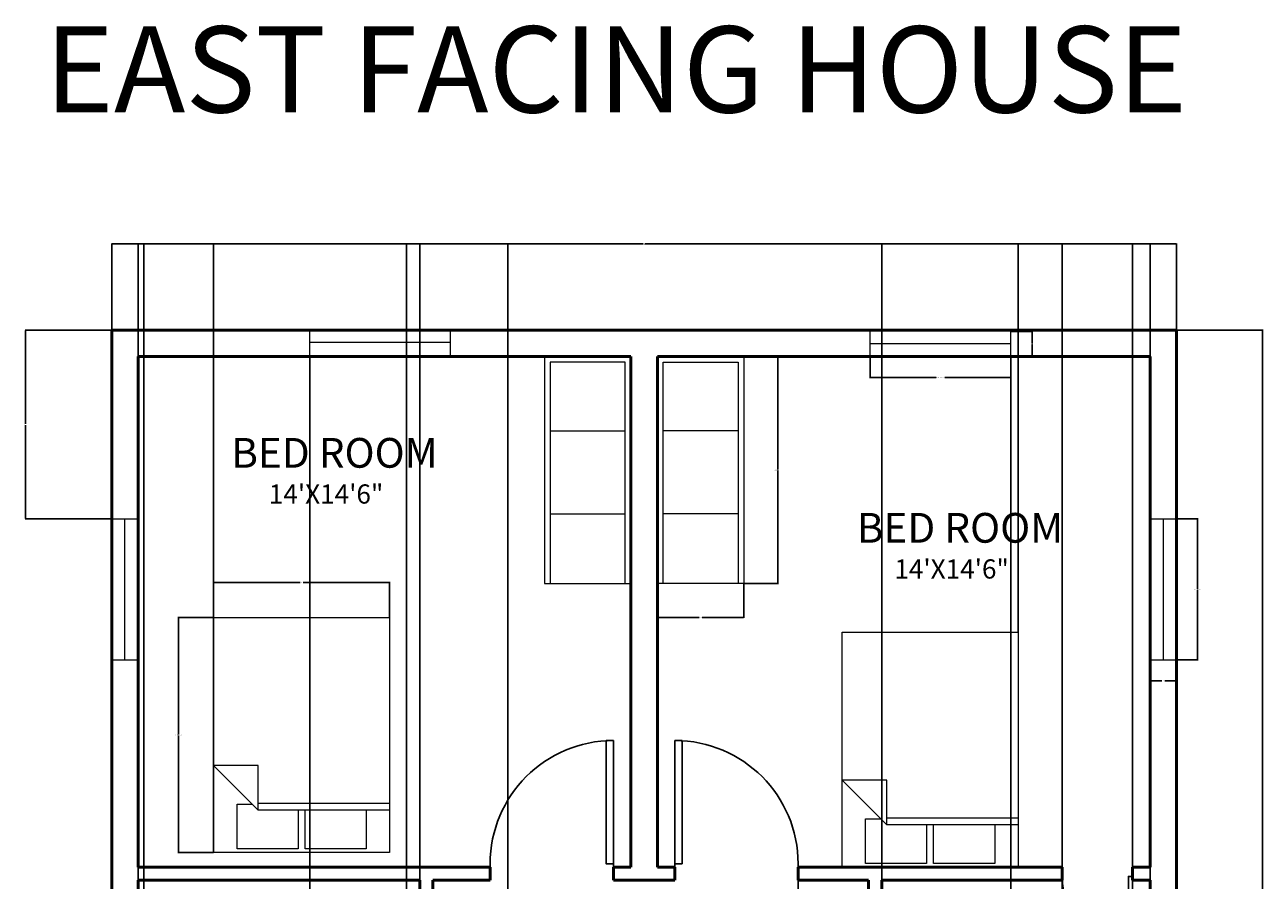
# Model space of a CAD drawing. Units: inches. Extents: x 19425 to 19848, y 45806 to 46417.
# Tile 5 of 5: x 19425 to 19847, y 46125 to 46417. Entities that reach past the tile are written whole.
import ezdxf

# ---------------------------------------------------------------- set-up
doc = ezdxf.new("R2010")
doc.units = ezdxf.units.IN
for name, color, linetype, lineweight in [('A-ANNO-DIMS', 2, 'Continuous', 18), ('A-ANNO-TITL', 7, 'Continuous', 35), ('A-AREA-IDEN', 3, 'Continuous', 25), ('A-FLOR-CASE', 2, 'Continuous', 20), ('door', 4, 'Continuous', 25), ('furniture', 2, 'Continuous', 18), ('wall', 6, 'Continuous', 50), ('window', 9, 'Continuous', 20)]:
    doc.layers.add(name, color=color, linetype=linetype, lineweight=lineweight)
doc.styles.get("Standard").update_dxf_attribs({"font": 'arial.ttf'})
doc.dimstyles.get("Standard").update_dxf_attribs({"dimtxt": 0.18, "dimasz": 0.18, "dimexe": 0.18, "dimexo": 0.0625, "dimgap": 0.09, "dimtad": 0, "dimtih": 1, "dimtoh": 1, "dimdec": 4, "dimzin": 0, "dimdsep": 46, "dimtxsty": 'Standard', "dimcen": 0.09, "dimadec": 0, "dimazin": 0, "dimtfac": 1, "dimtdec": 4, "dimtofl": 0, "dimtmove": 0, "dimatfit": 3, "dimfxl": 1, "dimtolj": 1, "dimtzin": 0, "dimarcsym": 0})

# ---------------------------------------------------------------- blocks, each defined once
blk = doc.blocks.new('*U2')
for p, q in [((0, 0), (0, -100)), ((750, 0), (750, -100))]:
    blk.add_line(p, q)
blk.add_lwpolyline([(0, 0), (0, 750), (43.75, 750), (43.75, 0)], close=True)
blk.add_arc((0, 0), 750, 0, 90)
blk = doc.blocks.new('Bed - Queen')
for p, q in [((0, -80.00003), (0, 0)), ((0, 0), (59.99999, 0)), ((59.99999, 0), (59.99999, -80.00003)), ((7.99999, -1.2), (28.79998, -1.2)), ((7.99999, -14.4), (7.99999, -1.2)), ((28.79998, -1.2), (28.79998, -14.4)), ((31.19999, -1.2), (51.99999, -1.2)), ((31.19999, -14.4), (31.19999, -1.2)), ((51.99999, -1.2), (51.99999, -16.4)), ((0, -14.4), (44.8, -14.4)), ((44.8, -16.8), (0, -16.8)), ((59.99999, -29.6), (44.8, -14.4)), ((44.8, -14.4), (44.8, -29.6)), ((51.99999, -16.4), (46.79936, -16.4)), ((44.8, -29.6), (59.99999, -29.6)), ((59.99999, -80.00003), (0, -80.00003))]:
    blk.add_line(p, q)
blk = doc.blocks.new('WIN-48-CENTER-9')
for p, q in [((0, 48), (9, 48)), ((4.5, 0), (4.5, 48)), ((0, 0), (9, 0))]:
    blk.add_line(p, q)
blk = doc.blocks.new('WIN-48-SHALLOW')
for p, q in [((0, 0), (0, 8.56)), ((48, 0), (48, 8.56)), ((48, 4.28), (0, 4.28))]:
    blk.add_line(p, q)
blk = doc.blocks.new('BEDROOM-WARDROBE')
for p, q in [((27.51, 52), (2, 52)), ((27.51, 23.7), (2, 23.7))]:
    blk.add_line(p, q)
blk.add_lwpolyline([(0, 77.33), (29.51, 77.33), (29.51, 0), (0, 0)], close=True)
blk.add_lwpolyline([(2, 0), (2, 75.33), (27.51, 75.33), (27.51, 0)])
blk = doc.blocks.new('*D16')
at = {"layer": 'A-ANNO-DIMS', "color": 0, "lineweight": -2, "transparency": 16777216}
for p, q in [((19817.84, 46248.39), (19825.16, 46248.39)), ((19824.98, 46248.21), (19824.98, 46224.57)), ((19824.98, 46200.57), (19824.98, 46224.2)), ((19817.84, 46200.39), (19825.16, 46200.39))]:
    blk.add_line(p, q, dxfattribs=at)
at = {"layer": 'A-ANNO-DIMS', "color": 0, "transparency": 16777216}
for points in [[(19824.95, 46248.21), (19825.01, 46248.21), (19824.98, 46248.39)], [(19824.95, 46200.57), (19825.01, 46200.57), (19824.98, 46200.39)]]:
    blk.add_solid(points, dxfattribs=at)
at = {"layer": 'Defpoints', "color": 0, "transparency": 16777216}
for p in [(19817.78, 46248.39), (19824.98, 46248.39), (19817.78, 46200.39)]:
    blk.add_point(p, dxfattribs=at)
at = {"layer": 'A-ANNO-DIMS', "color": 0, "transparency": 16777216, "insert": (19824.98, 46224.39), "char_height": 0.18, "attachment_point": 5}
blk.add_mtext('\\A1;SIDE WINDOW 48 TYP.', dxfattribs=at)
blk = doc.blocks.new('*D17')
at = {"layer": 'A-ANNO-DIMS', "color": 0, "lineweight": -2, "transparency": 16777216}
for p, q in [((19808.78, 46200.32), (19808.78, 46193.01)), ((19817.78, 46200.32), (19817.78, 46193.01)), ((19808.96, 46193.19), (19812.82, 46193.19)), ((19817.6, 46193.19), (19813.74, 46193.19))]:
    blk.add_line(p, q, dxfattribs=at)
at = {"layer": 'A-ANNO-DIMS', "color": 0, "transparency": 16777216}
for points in [[(19808.96, 46193.22), (19808.96, 46193.16), (19808.78, 46193.19)], [(19817.6, 46193.22), (19817.6, 46193.16), (19817.78, 46193.19)]]:
    blk.add_solid(points, dxfattribs=at)
at = {"layer": 'Defpoints', "color": 0, "transparency": 16777216}
for p in [(19808.78, 46200.39), (19817.78, 46200.39), (19817.78, 46193.19)]:
    blk.add_point(p, dxfattribs=at)
at = {"layer": 'A-ANNO-DIMS', "color": 0, "transparency": 16777216, "insert": (19813.28, 46193.19), "char_height": 0.18, "attachment_point": 5}
blk.add_mtext('\\A1;9 TYP.', dxfattribs=at)
blk = doc.blocks.new('*D20')
at = {"layer": 'A-ANNO-DIMS', "color": 0, "lineweight": -2, "transparency": 16777216}
for p, q in [((19489.43, 46214.75), (19477.32, 46214.75)), ((19477.5, 46214.57), (19477.5, 46174.94)), ((19477.5, 46134.93), (19477.5, 46174.56)), ((19489.43, 46134.75), (19477.32, 46134.75))]:
    blk.add_line(p, q, dxfattribs=at)
at = {"layer": 'A-ANNO-DIMS', "color": 0, "transparency": 16777216}
for points in [[(19477.47, 46214.57), (19477.53, 46214.57), (19477.5, 46214.75)], [(19477.47, 46134.93), (19477.53, 46134.93), (19477.5, 46134.75)]]:
    blk.add_solid(points, dxfattribs=at)
at = {"layer": 'Defpoints', "color": 0, "transparency": 16777216}
for p in [(19489.5, 46214.75), (19477.5, 46134.75), (19489.5, 46134.75)]:
    blk.add_point(p, dxfattribs=at)
at = {"layer": 'A-ANNO-DIMS', "color": 0, "transparency": 16777216, "insert": (19477.5, 46174.75), "char_height": 0.18, "attachment_point": 5}
blk.add_mtext('\\A1;QUEEN BED 80 TYP.', dxfattribs=at)
blk = doc.blocks.new('*D21')
at = {"layer": 'A-ANNO-DIMS', "color": 0, "lineweight": -2, "transparency": 16777216}
for p, q in [((19489.5, 46214.81), (19489.5, 46226.93)), ((19489.68, 46226.75), (19518.97, 46226.75)), ((19549.32, 46226.75), (19520.03, 46226.75)), ((19549.5, 46214.81), (19549.5, 46226.93))]:
    blk.add_line(p, q, dxfattribs=at)
at = {"layer": 'A-ANNO-DIMS', "color": 0, "transparency": 16777216}
for points in [[(19489.68, 46226.78), (19489.68, 46226.72), (19489.5, 46226.75)], [(19549.32, 46226.78), (19549.32, 46226.72), (19549.5, 46226.75)]]:
    blk.add_solid(points, dxfattribs=at)
at = {"layer": 'Defpoints', "color": 0, "transparency": 16777216}
for p in [(19489.5, 46226.75), (19489.5, 46214.75), (19549.5, 46214.75)]:
    blk.add_point(p, dxfattribs=at)
at = {"layer": 'A-ANNO-DIMS', "color": 0, "transparency": 16777216, "insert": (19519.5, 46226.75), "char_height": 0.18, "attachment_point": 5}
blk.add_mtext('\\A1;60 TYP.', dxfattribs=at)
blk = doc.blocks.new('*D22')
at = {"layer": 'A-ANNO-DIMS', "color": 0, "lineweight": -2, "transparency": 16777216}
for p, q in [((19713.31, 46303.69), (19713.31, 46296.37)), ((19761.31, 46303.69), (19761.31, 46296.37)), ((19713.49, 46296.55), (19735.81, 46296.55)), ((19761.13, 46296.55), (19738.8, 46296.55))]:
    blk.add_line(p, q, dxfattribs=at)
at = {"layer": 'A-ANNO-DIMS', "color": 0, "transparency": 16777216}
for points in [[(19713.49, 46296.58), (19713.49, 46296.52), (19713.31, 46296.55)], [(19761.13, 46296.58), (19761.13, 46296.52), (19761.31, 46296.55)]]:
    blk.add_solid(points, dxfattribs=at)
at = {"layer": 'Defpoints', "color": 0, "transparency": 16777216}
for p in [(19713.31, 46303.75), (19761.31, 46303.75), (19761.31, 46296.55)]:
    blk.add_point(p, dxfattribs=at)
at = {"layer": 'A-ANNO-DIMS', "color": 0, "transparency": 16777216, "insert": (19737.31, 46296.55), "char_height": 0.18, "attachment_point": 5}
blk.add_mtext('\\A1;REAR WINDOW 48 TYP.', dxfattribs=at)
blk = doc.blocks.new('*D23')
at = {"layer": 'A-ANNO-DIMS', "color": 0, "lineweight": -2, "transparency": 16777216}
for p, q in [((19761.37, 46312.31), (19768.69, 46312.31)), ((19768.51, 46312.13), (19768.51, 46308.21)), ((19768.51, 46303.93), (19768.51, 46307.85)), ((19761.37, 46303.75), (19768.69, 46303.75))]:
    blk.add_line(p, q, dxfattribs=at)
at = {"layer": 'A-ANNO-DIMS', "color": 0, "transparency": 16777216}
for points in [[(19768.48, 46312.13), (19768.54, 46312.13), (19768.51, 46312.31)], [(19768.48, 46303.93), (19768.54, 46303.93), (19768.51, 46303.75)]]:
    blk.add_solid(points, dxfattribs=at)
at = {"layer": 'Defpoints', "color": 0, "transparency": 16777216}
for p in [(19761.31, 46312.31), (19768.51, 46312.31), (19761.31, 46303.75)]:
    blk.add_point(p, dxfattribs=at)
at = {"layer": 'A-ANNO-DIMS', "color": 0, "transparency": 16777216, "insert": (19768.51, 46308.03), "char_height": 0.18, "attachment_point": 5}
blk.add_mtext('\\A1;9 TYP.', dxfattribs=at)
blk = doc.blocks.new('*D26')
at = {"layer": 'A-ANNO-DIMS', "color": 0, "lineweight": -2, "transparency": 16777216}
for p, q in [((19670.36, 46303.75), (19682.07, 46303.75)), ((19681.89, 46303.57), (19681.89, 46265.27)), ((19681.89, 46226.61), (19681.89, 46264.91)), ((19670.36, 46226.43), (19682.07, 46226.43))]:
    blk.add_line(p, q, dxfattribs=at)
at = {"layer": 'A-ANNO-DIMS', "color": 0, "transparency": 16777216}
for points in [[(19681.86, 46303.57), (19681.92, 46303.57), (19681.89, 46303.75)], [(19681.86, 46226.61), (19681.92, 46226.61), (19681.89, 46226.43)]]:
    blk.add_solid(points, dxfattribs=at)
at = {"layer": 'Defpoints', "color": 0, "transparency": 16777216}
for p in [(19670.3, 46303.75), (19681.89, 46303.75), (19670.3, 46226.43)]:
    blk.add_point(p, dxfattribs=at)
at = {"layer": 'A-ANNO-DIMS', "color": 0, "transparency": 16777216, "insert": (19681.89, 46265.09), "char_height": 0.18, "attachment_point": 5}
blk.add_mtext('\\A1;WARDROBE 77 TYP.', dxfattribs=at)
blk = doc.blocks.new('*D27')
at = {"layer": 'A-ANNO-DIMS', "color": 0, "lineweight": -2, "transparency": 16777216}
for p, q in [((19640.78, 46226.37), (19640.78, 46214.65)), ((19670.3, 46226.37), (19670.3, 46214.65)), ((19640.96, 46214.83), (19655.01, 46214.83)), ((19670.12, 46214.83), (19656.07, 46214.83))]:
    blk.add_line(p, q, dxfattribs=at)
at = {"layer": 'A-ANNO-DIMS', "color": 0, "transparency": 16777216}
for points in [[(19640.96, 46214.86), (19640.96, 46214.8), (19640.78, 46214.83)], [(19670.12, 46214.86), (19670.12, 46214.8), (19670.3, 46214.83)]]:
    blk.add_solid(points, dxfattribs=at)
at = {"layer": 'Defpoints', "color": 0, "transparency": 16777216}
for p in [(19640.78, 46226.43), (19670.3, 46226.43), (19670.3, 46214.83)]:
    blk.add_point(p, dxfattribs=at)
at = {"layer": 'A-ANNO-DIMS', "color": 0, "transparency": 16777216, "insert": (19655.54, 46214.83), "char_height": 0.18, "attachment_point": 5}
blk.add_mtext('\\A1;30 TYP.', dxfattribs=at)
blk = doc.blocks.new('*D32')
at = {"layer": 'A-ANNO-DIMS', "color": 0, "lineweight": -2, "transparency": 16777216}
for p, q in [((19454.78, 46312.82), (19454.78, 46342.28)), ((19454.96, 46342.1), (19635.99, 46342.1)), ((19817.6, 46342.1), (19636.57, 46342.1)), ((19817.78, 46312.82), (19817.78, 46342.28))]:
    blk.add_line(p, q, dxfattribs=at)
at = {"layer": 'A-ANNO-DIMS', "color": 0, "transparency": 16777216}
for points in [[(19454.96, 46342.13), (19454.96, 46342.07), (19454.78, 46342.1)], [(19817.6, 46342.13), (19817.6, 46342.07), (19817.78, 46342.1)]]:
    blk.add_solid(points, dxfattribs=at)
at = {"layer": 'Defpoints', "color": 0, "transparency": 16777216}
for p in [(19817.78, 46342.1), (19454.78, 46312.75), (19817.78, 46312.75)]:
    blk.add_point(p, dxfattribs=at)
at = {"layer": 'A-ANNO-DIMS', "color": 0, "transparency": 16777216, "insert": (19636.28, 46342.1), "char_height": 0.18, "attachment_point": 5}
blk.add_mtext('\\A1;363', dxfattribs=at)
blk = doc.blocks.new('*D33')
at = {"layer": 'A-ANNO-DIMS', "color": 0, "lineweight": -2, "transparency": 16777216}
for p, q in [((19817.843662, 46312.754651), (19847.311162, 46312.754651)), ((19847.131162, 46312.574651), (19847.131162, 46074.434651)), ((19847.131162, 45835.934651), (19847.131162, 46074.074651)), ((19817.843662, 45835.754651), (19847.311162, 45835.754651))]:
    blk.add_line(p, q, dxfattribs=at)
at = {"layer": 'A-ANNO-DIMS', "color": 0, "transparency": 16777216}
for points in [[(19847.101162, 46312.574651), (19847.161162, 46312.574651), (19847.131162, 46312.754651)], [(19847.101162, 45835.934651), (19847.161162, 45835.934651), (19847.131162, 45835.754651)]]:
    blk.add_solid(points, dxfattribs=at)
at = {"layer": 'Defpoints', "color": 0, "transparency": 16777216}
for p in [(19817.781162, 46312.754651), (19847.131162, 46312.754651), (19817.781162, 45835.754651)]:
    blk.add_point(p, dxfattribs=at)
at = {"layer": 'A-ANNO-DIMS', "color": 0, "transparency": 16777216, "insert": (19847.131162, 46074.254651), "char_height": 0.18, "attachment_point": 5}
blk.add_mtext('\\A1;477', dxfattribs=at)
blk = doc.blocks.new('*D34')
at = {"layer": 'A-ANNO-DIMS', "color": 0, "lineweight": -2, "transparency": 16777216}
for p, q in [((19522.3, 46304.14), (19522.3, 45806.22)), ((19463.78, 46303.69), (19463.78, 45806.22)), ((19463.96, 45806.4), (19492.65, 45806.4)), ((19522.12, 45806.4), (19493.43, 45806.4))]:
    blk.add_line(p, q, dxfattribs=at)
at = {"layer": 'A-ANNO-DIMS', "color": 0, "transparency": 16777216}
for points in [[(19463.96, 45806.43), (19463.96, 45806.37), (19463.78, 45806.4)], [(19522.12, 45806.43), (19522.12, 45806.37), (19522.3, 45806.4)]]:
    blk.add_solid(points, dxfattribs=at)
at = {"layer": 'Defpoints', "color": 0, "transparency": 16777216}
for p in [(19522.3, 46304.2), (19463.78, 46303.75), (19522.3, 45806.4)]:
    blk.add_point(p, dxfattribs=at)
at = {"layer": 'A-ANNO-DIMS', "color": 0, "transparency": 16777216, "insert": (19493.04, 45806.4), "char_height": 0.18, "attachment_point": 5}
blk.add_mtext('\\A1;58.52', dxfattribs=at)
blk = doc.blocks.new('*D35')
at = {"layer": 'A-ANNO-DIMS', "color": 0, "lineweight": -2, "transparency": 16777216}
for p, q in [((19761.31, 46303.69), (19761.31, 45806.22)), ((19808.78, 46303.69), (19808.78, 45806.22)), ((19761.49, 45806.4), (19784.65, 45806.4)), ((19808.6, 45806.4), (19785.44, 45806.4))]:
    blk.add_line(p, q, dxfattribs=at)
at = {"layer": 'A-ANNO-DIMS', "color": 0, "transparency": 16777216}
for points in [[(19761.49, 45806.43), (19761.49, 45806.37), (19761.31, 45806.4)], [(19808.6, 45806.43), (19808.6, 45806.37), (19808.78, 45806.4)]]:
    blk.add_solid(points, dxfattribs=at)
at = {"layer": 'Defpoints', "color": 0, "transparency": 16777216}
for p in [(19761.31, 46303.75), (19808.78, 46303.75), (19808.78, 45806.4)]:
    blk.add_point(p, dxfattribs=at)
at = {"layer": 'A-ANNO-DIMS', "color": 0, "transparency": 16777216, "insert": (19785.04, 45806.4), "char_height": 0.18, "attachment_point": 5}
blk.add_mtext('\\A1;47.47', dxfattribs=at)
blk = doc.blocks.new('*D36')
at = {"layer": 'A-ANNO-DIMS', "color": 0, "lineweight": -2, "transparency": 16777216}
for p, q in [((19454.72, 46312.75), (19425.25, 46312.75)), ((19425.43, 46312.57), (19425.43, 46280.75)), ((19425.43, 46248.57), (19425.43, 46280.39)), ((19454.72, 46248.39), (19425.25, 46248.39))]:
    blk.add_line(p, q, dxfattribs=at)
at = {"layer": 'A-ANNO-DIMS', "color": 0, "transparency": 16777216}
for points in [[(19425.4, 46312.57), (19425.46, 46312.57), (19425.43, 46312.75)], [(19425.4, 46248.57), (19425.46, 46248.57), (19425.43, 46248.39)]]:
    blk.add_solid(points, dxfattribs=at)
at = {"layer": 'Defpoints', "color": 0, "transparency": 16777216}
for p in [(19454.78, 46312.75), (19425.43, 46248.39), (19454.78, 46248.39)]:
    blk.add_point(p, dxfattribs=at)
at = {"layer": 'A-ANNO-DIMS', "color": 0, "transparency": 16777216, "insert": (19425.43, 46280.57), "char_height": 0.18, "attachment_point": 5}
blk.add_mtext('\\A1;64.37', dxfattribs=at)
blk = doc.blocks.new('*D44')
at = {"layer": 'A-ANNO-DIMS', "color": 0, "lineweight": -2, "transparency": 16777216}
for p, q in [((19463.78, 45969.32), (19463.78, 46342.28)), ((19463.96, 46342.1), (19526.5, 46342.1)), ((19589.6, 46342.1), (19527.06, 46342.1)), ((19589.78, 45969.32), (19589.78, 46342.28))]:
    blk.add_line(p, q, dxfattribs=at)
at = {"layer": 'A-ANNO-DIMS', "color": 0, "transparency": 16777216}
for points in [[(19463.96, 46342.13), (19463.96, 46342.07), (19463.78, 46342.1)], [(19589.6, 46342.13), (19589.6, 46342.07), (19589.78, 46342.1)]]:
    blk.add_solid(points, dxfattribs=at)
at = {"layer": 'Defpoints', "color": 0, "transparency": 16777216}
for p in [(19589.78, 46342.1), (19463.78, 45969.25), (19589.78, 45969.25)]:
    blk.add_point(p, dxfattribs=at)
at = {"layer": 'A-ANNO-DIMS', "color": 0, "transparency": 16777216, "insert": (19526.78, 46342.1), "char_height": 0.18, "attachment_point": 5}
blk.add_mtext('\\A1;126', dxfattribs=at)
blk = doc.blocks.new('*D47')
at = {"layer": 'A-ANNO-DIMS', "color": 0, "lineweight": -2, "transparency": 16777216}
for p, q in [((19778.78, 46129.82), (19778.78, 46342.28)), ((19778.96, 46342.1), (19790.56, 46342.1)), ((19802.6, 46342.1), (19791, 46342.1)), ((19802.78, 46129.82), (19802.78, 46342.28))]:
    blk.add_line(p, q, dxfattribs=at)
at = {"layer": 'A-ANNO-DIMS', "color": 0, "transparency": 16777216}
for points in [[(19778.96, 46342.13), (19778.96, 46342.07), (19778.78, 46342.1)], [(19802.6, 46342.13), (19802.6, 46342.07), (19802.78, 46342.1)]]:
    blk.add_solid(points, dxfattribs=at)
at = {"layer": 'Defpoints', "color": 0, "transparency": 16777216}
for p in [(19802.78, 46342.1), (19778.78, 46129.75), (19802.78, 46129.75)]:
    blk.add_point(p, dxfattribs=at)
at = {"layer": 'A-ANNO-DIMS', "color": 0, "transparency": 16777216, "insert": (19790.78, 46342.1), "char_height": 0.18, "attachment_point": 5}
blk.add_mtext('\\A1;24', dxfattribs=at)
blk = doc.blocks.new('*D55')
at = {"layer": 'A-ANNO-DIMS', "color": 0, "lineweight": -2, "transparency": 16777216}
for p, q in [((19717.28, 46053.32), (19717.28, 46342.28)), ((19717.46, 46342.1), (19762.71, 46342.1)), ((19808.6, 46342.1), (19763.36, 46342.1)), ((19808.78, 46053.32), (19808.78, 46342.28))]:
    blk.add_line(p, q, dxfattribs=at)
at = {"layer": 'A-ANNO-DIMS', "color": 0, "transparency": 16777216}
for points in [[(19717.46, 46342.13), (19717.46, 46342.07), (19717.28, 46342.1)], [(19808.6, 46342.13), (19808.6, 46342.07), (19808.78, 46342.1)]]:
    blk.add_solid(points, dxfattribs=at)
at = {"layer": 'Defpoints', "color": 0, "transparency": 16777216}
for p in [(19808.78, 46342.1), (19717.28, 46053.25), (19808.78, 46053.25)]:
    blk.add_point(p, dxfattribs=at)
at = {"layer": 'A-ANNO-DIMS', "color": 0, "transparency": 16777216, "insert": (19763.03, 46342.1), "char_height": 0.18, "attachment_point": 5}
blk.add_mtext('\\A1;91.5', dxfattribs=at)
blk = doc.blocks.new('*D59')
at = {"layer": 'A-ANNO-DIMS', "color": 0, "lineweight": -2, "transparency": 16777216}
for p, q in [((19463.78, 45868.98), (19463.78, 46342.28)), ((19463.96, 46342.1), (19464.36, 46342.1)), ((19465.54, 46342.1), (19465.14, 46342.1)), ((19465.72, 45866.97), (19465.72, 46342.28))]:
    blk.add_line(p, q, dxfattribs=at)
at = {"layer": 'A-ANNO-DIMS', "color": 0, "transparency": 16777216}
for points in [[(19463.96, 46342.13), (19463.96, 46342.07), (19463.78, 46342.1)], [(19465.54, 46342.13), (19465.54, 46342.07), (19465.72, 46342.1)]]:
    blk.add_solid(points, dxfattribs=at)
at = {"layer": 'Defpoints', "color": 0, "transparency": 16777216}
for p in [(19465.72, 46342.1), (19463.78, 45868.92), (19465.72, 45866.91)]:
    blk.add_point(p, dxfattribs=at)
at = {"layer": 'A-ANNO-DIMS', "color": 0, "transparency": 16777216, "insert": (19464.75, 46342.1), "char_height": 0.18, "attachment_point": 5}
blk.add_mtext('\\A1;1.938', dxfattribs=at)
blk = doc.blocks.new('*D60')
at = {"layer": 'A-ANNO-DIMS', "color": 0, "lineweight": -2, "transparency": 16777216}
for p, q in [((19555.24, 45865.14), (19555.24, 46342.28)), ((19555.42, 46342.1), (19557.18, 46342.1)), ((19559.6, 46342.1), (19557.84, 46342.1)), ((19559.78, 45868.98), (19559.78, 46342.28))]:
    blk.add_line(p, q, dxfattribs=at)
at = {"layer": 'A-ANNO-DIMS', "color": 0, "transparency": 16777216}
for points in [[(19555.42, 46342.13), (19555.42, 46342.07), (19555.24, 46342.1)], [(19559.6, 46342.13), (19559.6, 46342.07), (19559.78, 46342.1)]]:
    blk.add_solid(points, dxfattribs=at)
at = {"layer": 'Defpoints', "color": 0, "transparency": 16777216}
for p in [(19559.78, 46342.1), (19555.24, 45865.08), (19559.78, 45868.92)]:
    blk.add_point(p, dxfattribs=at)
at = {"layer": 'A-ANNO-DIMS', "color": 0, "transparency": 16777216, "insert": (19557.51, 46342.1), "char_height": 0.18, "attachment_point": 5}
blk.add_mtext('\\A1;4.54', dxfattribs=at)
blk = doc.blocks.new('*D61')
at = {"layer": 'A-ANNO-DIMS', "color": 0, "lineweight": -2, "transparency": 16777216}
for p, q in [((19463.78, 46129.82), (19463.78, 46342.28)), ((19463.96, 46342.1), (19476.17, 46342.1)), ((19489.32, 46342.1), (19477.1, 46342.1)), ((19489.5, 46134.81), (19489.5, 46342.28))]:
    blk.add_line(p, q, dxfattribs=at)
at = {"layer": 'A-ANNO-DIMS', "color": 0, "transparency": 16777216}
for points in [[(19463.96, 46342.13), (19463.96, 46342.07), (19463.78, 46342.1)], [(19489.32, 46342.13), (19489.32, 46342.07), (19489.5, 46342.1)]]:
    blk.add_solid(points, dxfattribs=at)
at = {"layer": 'Defpoints', "color": 0, "transparency": 16777216}
for p in [(19489.5, 46342.1), (19489.5, 46134.75), (19463.78, 46129.75)]:
    blk.add_point(p, dxfattribs=at)
at = {"layer": 'A-ANNO-DIMS', "color": 0, "transparency": 16777216, "insert": (19476.64, 46342.1), "char_height": 0.18, "attachment_point": 5}
blk.add_mtext('\\A1;25.715', dxfattribs=at)
blk = doc.blocks.new('*D62')
at = {"layer": 'A-ANNO-DIMS', "color": 0, "lineweight": -2, "transparency": 16777216}
for p, q in [((19763.78, 46209.82), (19763.78, 46342.28)), ((19763.96, 46342.1), (19786.06, 46342.1)), ((19808.6, 46342.1), (19786.5, 46342.1)), ((19808.78, 46200.45), (19808.78, 46342.28))]:
    blk.add_line(p, q, dxfattribs=at)
at = {"layer": 'A-ANNO-DIMS', "color": 0, "transparency": 16777216}
for points in [[(19763.96, 46342.13), (19763.96, 46342.07), (19763.78, 46342.1)], [(19808.6, 46342.13), (19808.6, 46342.07), (19808.78, 46342.1)]]:
    blk.add_solid(points, dxfattribs=at)
at = {"layer": 'Defpoints', "color": 0, "transparency": 16777216}
for p in [(19808.78, 46342.1), (19763.78, 46209.75), (19808.78, 46200.39)]:
    blk.add_point(p, dxfattribs=at)
at = {"layer": 'A-ANNO-DIMS', "color": 0, "transparency": 16777216, "insert": (19786.28, 46342.1), "char_height": 0.18, "attachment_point": 5}
blk.add_mtext('\\A1;45', dxfattribs=at)
blk = doc.blocks.new('*D74')
at = {"layer": 'A-ANNO-DIMS', "color": 0, "lineweight": -2, "transparency": 16777216}
for p, q in [((19688.78, 46129.69), (19688.78, 45806.22)), ((19778.78, 46129.69), (19778.78, 45806.22)), ((19688.96, 45806.4), (19733.56, 45806.4)), ((19778.6, 45806.4), (19734, 45806.4))]:
    blk.add_line(p, q, dxfattribs=at)
at = {"layer": 'A-ANNO-DIMS', "color": 0, "transparency": 16777216}
for points in [[(19688.96, 45806.43), (19688.96, 45806.37), (19688.78, 45806.4)], [(19778.6, 45806.43), (19778.6, 45806.37), (19778.78, 45806.4)]]:
    blk.add_solid(points, dxfattribs=at)
at = {"layer": 'Defpoints', "color": 0, "transparency": 16777216}
for p in [(19688.78, 46129.75), (19778.78, 46129.75), (19778.78, 45806.4)]:
    blk.add_point(p, dxfattribs=at)
at = {"layer": 'A-ANNO-DIMS', "color": 0, "transparency": 16777216, "insert": (19733.78, 45806.4), "char_height": 0.18, "attachment_point": 5}
blk.add_mtext('\\A1;90', dxfattribs=at)

msp = doc.modelspace()

# ---------------------------------------------------------------- linework, layer by layer
at = {"layer": 'wall'}
for p, q in [((19454.7812, 46312.7547), (19817.7812, 46312.7547)), ((19454.7812, 46312.7547), (19454.7812, 45835.7547)), ((19817.7812, 46312.7547), (19817.7812, 45835.7547)), ((19463.7812, 46303.7547), (19463.7812, 46129.7547)), ((19463.7812, 46303.7547), (19631.7812, 46303.7547)), ((19631.7812, 46303.7547), (19631.7812, 46129.7547)), ((19640.7812, 46303.7547), (19640.7812, 46129.7547)), ((19640.7812, 46303.7547), (19808.7812, 46303.7547)), ((19808.7812, 46303.7547), (19808.7812, 46129.7547)), ((19463.7812, 46129.7547), (19583.7812, 46129.7547)), ((19583.7812, 46129.7547), (19583.7812, 46125.2547)), ((19625.7812, 46129.7547), (19625.7812, 46125.2547)), ((19625.7812, 46129.7547), (19631.7812, 46129.7547)), ((19640.7812, 46129.7547), (19646.7812, 46129.7547)), ((19646.7812, 46129.7547), (19646.7812, 46125.2547)), ((19688.7812, 46129.7547), (19688.7812, 46125.2547)), ((19688.7812, 46129.7547), (19778.7812, 46129.7547)), ((19778.7812, 46129.7547), (19778.7812, 46125.2547)), ((19802.7812, 46129.7547), (19802.7812, 46125.2547)), ((19802.7812, 46129.7547), (19808.7812, 46129.7547)), ((19463.7812, 46125.2547), (19559.7812, 46125.2547)), ((19463.7812, 46125.2547), (19463.7812, 46053.2547)), ((19559.7812, 46125.2547), (19559.7812, 46119.2547)), ((19564.2812, 46125.2547), (19564.2812, 46119.2547)), ((19564.2812, 46125.2547), (19583.7812, 46125.2547)), ((19625.7812, 46125.2547), (19646.7812, 46125.2547)), ((19688.7812, 46125.2547), (19712.7812, 46125.2547)), ((19712.7812, 46125.2547), (19712.7812, 46048.7547)), ((19717.2812, 46125.2547), (19717.2812, 46053.2547)), ((19717.2812, 46125.2547), (19778.7812, 46125.2547)), ((19802.7812, 46125.2547), (19808.7812, 46125.2547)), ((19808.7812, 46125.2547), (19808.7812, 46053.2547))]:
    msp.add_line(p, q, dxfattribs=at)

# ---------------------------------------------------------------- block references
at = {"layer": 'A-FLOR-CASE', "extrusion": (0, 0, -1), "zscale": -1}
msp.add_blockref('BEDROOM-WARDROBE', (-19631.7812, 46226.4279), dxfattribs=at)
at = {"layer": 'A-FLOR-CASE'}
msp.add_blockref('BEDROOM-WARDROBE', (19640.7812, 46226.4279), dxfattribs=at)
at = {"layer": 'door', "yscale": 0.0560000000000015, "zscale": 0.0560000000000015}
for p, xscale in [((19625.7812, 46130.8547), -0.0560000000000015), ((19646.7812, 46130.8547), 0.0560000000000015)]:
    msp.add_blockref('*U2', p, dxfattribs=dict(at, xscale=xscale))
at = {"layer": 'door', "xscale": 0.0320000000000009, "yscale": 0.0320000000000009, "zscale": 0.0320000000000009, "rotation": 180}
msp.add_blockref('*U2', (19802.7812, 46126.5547), dxfattribs=at)
at = {"layer": 'furniture', "rotation": 180}
for p in [(19549.4966, 46134.7513), (19763.7812, 46129.7547)]:
    msp.add_blockref('Bed - Queen', p, dxfattribs=at)
at = {"layer": 'window'}
for name, p in [('WIN-48-SHALLOW', (19522.3015, 46304.1988)), ('WIN-48-SHALLOW', (19713.3082, 46303.7547)), ('WIN-48-CENTER-9', (19454.7812, 46200.3854)), ('WIN-48-CENTER-9', (19808.7812, 46200.3854))]:
    msp.add_blockref(name, p, dxfattribs=at)

# ---------------------------------------------------------------- texts
at = {"layer": 'A-ANNO-TITL'}
msp.add_text('EAST FACING HOUSE', height=29.373916, dxfattribs=at).set_placement((19431.9186, 46386.8965))
at = {"layer": 'A-AREA-IDEN'}
for s, height, p in [('BED ROOM', 10.12861, (19495.5456, 46265.8398)), ('14\'X14\'6"', 6.53608, (19508.3259, 46253.6138)), ('BED ROOM', 10.12861, (19708.8013, 46240.2881)), ('14\'X14\'6"', 6.53608, (19721.5816, 46228.0621))]:
    msp.add_text(s, height=height, dxfattribs=at).set_placement(p)

# ---------------------------------------------------------------- dimensions: what is measured, and where the dimension line sits
at = {"layer": 'A-ANNO-DIMS'}
for base, p1, p2, override, picture, middle in [((19817.7812, 46342.1047), (19454.7812, 46312.7547), (19817.7812, 46312.7547), {"dimdec": 0, "dimlfac": 1, "dimrnd": 0, "dimzin": 0, "dimdsep": 46, "dimlunit": 2}, '*D32', (19636.2812, 46342.1047)), ((19589.7812, 46342.1047), (19463.7812, 45969.2547), (19589.7812, 45969.2547), {"dimdec": 0, "dimlfac": 1, "dimrnd": 0, "dimzin": 0, "dimdsep": 46, "dimlunit": 2}, '*D44', (19526.7812, 46342.1047)), ((19465.7192, 46342.1047), (19463.7812, 45868.9163), (19465.7192, 45866.9088), {"dimdec": 3, "dimlfac": 1, "dimrnd": 0, "dimzin": 0, "dimdsep": 46, "dimlunit": 2}, '*D59', (19464.7502, 46342.1047)), ((19489.4966, 46342.1047), (19463.7812, 46129.7547), (19489.4966, 46134.7513), {"dimdec": 3, "dimlfac": 1, "dimrnd": 0, "dimzin": 0, "dimdsep": 46, "dimlunit": 2}, '*D61', (19476.6389, 46342.1047)), ((19559.7812, 46342.1047), (19555.2409, 45865.0758), (19559.7812, 45868.9163), {"dimdec": 2, "dimlfac": 1, "dimrnd": 0, "dimzin": 0, "dimdsep": 46, "dimlunit": 2}, '*D60', (19557.511, 46342.1047)), ((19808.7812, 46342.1047), (19717.2812, 46053.2547), (19808.7812, 46053.2547), {"dimdec": 1, "dimlfac": 1, "dimrnd": 0, "dimzin": 0, "dimdsep": 46, "dimlunit": 2}, '*D55', (19763.0312, 46342.1047)), ((19808.7812, 46342.1047), (19763.7812, 46209.7547), (19808.7812, 46200.3854), {"dimdec": 0, "dimlfac": 1, "dimrnd": 0, "dimzin": 0, "dimdsep": 46, "dimlunit": 2}, '*D62', (19786.2812, 46342.1047)), ((19802.7812, 46342.1047), (19778.7812, 46129.7547), (19802.7812, 46129.7547), {"dimdec": 0, "dimlfac": 1, "dimrnd": 0, "dimzin": 0, "dimdsep": 46, "dimlunit": 2}, '*D47', (19790.7812, 46342.1047)), ((19522.3015, 45806.4047), (19463.7812, 46303.7547), (19522.3015, 46304.1988), {"dimdec": 2, "dimlfac": 1, "dimrnd": 0, "dimzin": 0, "dimdsep": 46, "dimlunit": 2}, '*D34', (19493.0413, 45806.4047)), ((19808.7812, 45806.4047), (19761.3082, 46303.7547), (19808.7812, 46303.7547), {"dimdec": 2, "dimlfac": 1, "dimrnd": 0, "dimzin": 0, "dimdsep": 46, "dimlunit": 2}, '*D35', (19785.0447, 45806.4047)), ((19778.7812, 45806.4047), (19688.7812, 46129.7547), (19778.7812, 46129.7547), {"dimdec": 0, "dimlfac": 1, "dimrnd": 0, "dimzin": 0, "dimdsep": 46, "dimlunit": 2}, '*D74', (19733.7812, 45806.4047))]:
    dim = msp.add_linear_dim(base=base, p1=p1, p2=p2, dimstyle='Standard', override=override, dxfattribs=at)
    dim.commit()
    dim.dimension.update_dxf_attribs({"geometry": picture, "text_midpoint": middle})
for base, p1, p2, override, picture, middle in [((19425.4312, 46248.3854), (19454.7812, 46312.7547), (19454.7812, 46248.3854), {"dimdec": 2, "dimlfac": 1, "dimrnd": 0, "dimzin": 0, "dimdsep": 46, "dimlunit": 2}, '*D36', (19425.4312, 46280.57)), ((19847.1312, 46312.7547), (19817.7812, 45835.7547), (19817.7812, 46312.7547), {"dimdec": 0, "dimlfac": 1, "dimrnd": 0, "dimzin": 0, "dimdsep": 46, "dimlunit": 2}, '*D33', (19847.1312, 46074.2547))]:
    dim = msp.add_linear_dim(base=base, p1=p1, p2=p2, angle=90, dimstyle='Standard', override=override, dxfattribs=at)
    dim.commit()
    dim.dimension.update_dxf_attribs({"geometry": picture, "text_midpoint": middle})
for base, p1, p2, angle, text, picture, middle in [((19768.5082, 46312.3105), (19761.3082, 46303.7547), (19761.3082, 46312.3105), 90, '<> TYP.', '*D23', (19768.5082, 46308.0326)), ((19681.8944, 46303.7547), (19670.2954, 46226.4279), (19670.2954, 46303.7547), 90, 'WARDROBE <> TYP.', '*D26', (19681.8944, 46265.0913)), ((19824.9812, 46248.3854), (19817.7812, 46200.3854), (19817.7812, 46248.3854), 90, 'SIDE WINDOW <> TYP.', '*D16', (19824.9812, 46224.3854)), ((19489.4966, 46226.7514), (19549.4966, 46214.7514), (19489.4966, 46214.7514), 180, '<> TYP.', '*D21', (19519.4966, 46226.7514)), ((19477.4966, 46134.7513), (19489.4966, 46214.7514), (19489.4966, 46134.7513), 270, 'QUEEN BED <> TYP.', '*D20', (19477.4966, 46174.7514))]:
    dim = msp.add_linear_dim(base=base, p1=p1, p2=p2, angle=angle, text=text, dimstyle='Standard', override={"dimdec": 0, "dimlfac": 1, "dimrnd": 0, "dimzin": 0, "dimdsep": 46, "dimlunit": 2}, dxfattribs=at)
    dim.commit()
    dim.dimension.update_dxf_attribs({"geometry": picture, "text_midpoint": middle})
for base, p1, p2, text, picture, middle in [((19761.3082, 46296.5547), (19713.3082, 46303.7547), (19761.3082, 46303.7547), 'REAR WINDOW <> TYP.', '*D22', (19737.3082, 46296.5547)), ((19670.2954, 46214.8289), (19640.7812, 46226.4279), (19670.2954, 46226.4279), '<> TYP.', '*D27', (19655.5383, 46214.8289)), ((19817.7812, 46193.1854), (19808.7812, 46200.3854), (19817.7812, 46200.3854), '<> TYP.', '*D17', (19813.2812, 46193.1854))]:
    dim = msp.add_linear_dim(base=base, p1=p1, p2=p2, text=text, dimstyle='Standard', override={"dimdec": 0, "dimlfac": 1, "dimrnd": 0, "dimzin": 0, "dimdsep": 46, "dimlunit": 2}, dxfattribs=at)
    dim.commit()
    dim.dimension.update_dxf_attribs({"geometry": picture, "text_midpoint": middle})

doc.saveas('drawing.dxf')
